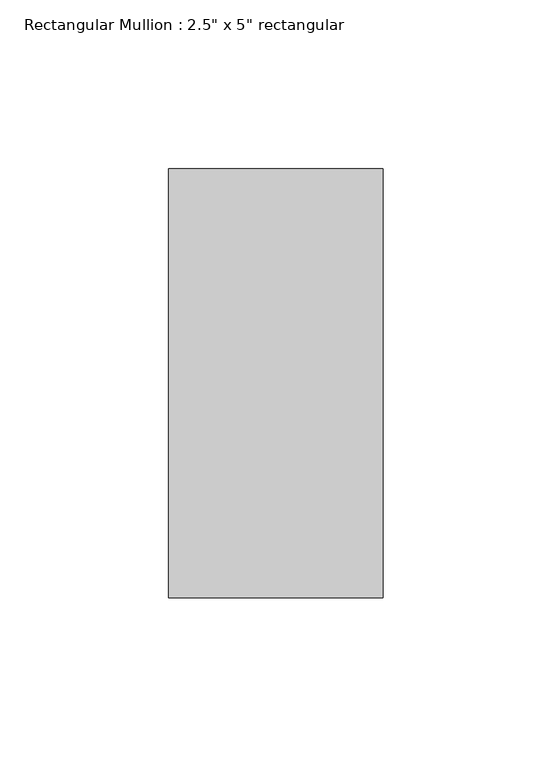
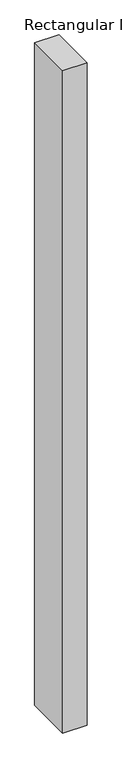
"""IFC4 building model written with IfcOpenShell, lengths in millimetres: member geometry."""

from ifc_helpers import new_model, si_unit, frame, origin, place, context, project, spatial, polyline, outline, extrude, source, transform, mapped, element, save


def member_d60e8053(model_context):
    return source(origin(), model_context, "Body", "SweptSolid", [
        extrude(outline(polyline([(31.75, 63.5), (31.75, -63.5), (-31.75, -63.5), (-31.75, 63.5), (31.75, 63.5)])), frame((0.0, 0.0, -1828.8), z_axis=(0.0, 0.0, 1.0), x_axis=(1.0, 0.0, 0.0)), (0.0, 0.0, 1.0), 1828.8),
    ])


if __name__ == "__main__":
    model = new_model("IFC4")
    model_context = context("Model", 3, world=origin())
    ifc_project = project(units=[si_unit("LENGTHUNIT", "METRE", prefix="MILLI")], contexts=[model_context])
    site = spatial("IfcSite", under=ifc_project)
    building = spatial("IfcBuilding", under=site)
    placement = place(None, origin())
    member_shape = member_d60e8053(model_context)
    element("IfcMember", 1, ObjectType="Rectangular Mullion : 2.5\" x 5\" rectangular", at=placement, inside=building, context=model_context, shape_type="MappedRepresentation", body=[
        mapped(member_shape, transform((0.0, 0.0, 0.0), x_axis=(1.0, 0.0, 0.0), y_axis=(0.0, 1.0, 0.0), z_axis=(0.0, 0.0, 1.0))),
    ])
    save(model, "model.ifc")

# Revit data of these elements
# Type "Rectangular Mullion : 2.5\" x 5\" rectangular"
#   built-in parameter 1007304 = 0.416667 (stored number, unit not read)
#   built-in parameter 1007301 = 0.104167 (stored number, unit not read)
#   built-in parameter 1007300 = 0.104167 (stored number, unit not read)
# Element 1 (IfcMember, "Rectangular Mullion : 2.5\" x 5\" rectangular")
#   Materials on its faces: "Aluminum"
# Materials
#   "Aluminum": class "Metal", colour RGB 247 247 247, transparency 0, Description = "Aluminum 6061", Cost = 0
